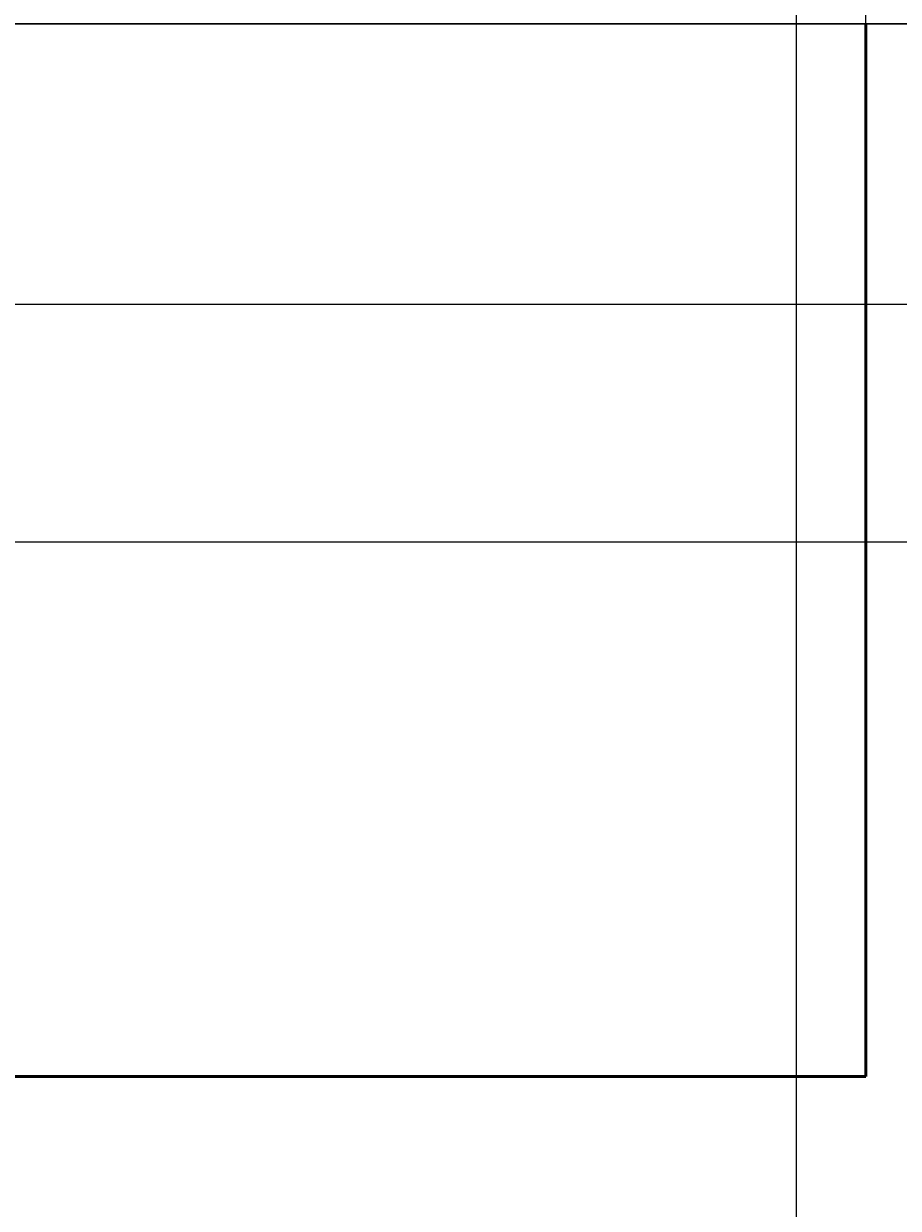
# Model space of a CAD drawing. Units: inches. Extents: x 37 to 824, y -700 to 234.
# Tile 64 of 77: x 314 to 364, y 8 to 75. Entities that reach past the tile are written whole.
import ezdxf

# ---------------------------------------------------------------- set-up
doc = ezdxf.new("R2010")
doc.units = ezdxf.units.IN
doc.header["$MEASUREMENT"] = 0
doc.layers.add('A-ANNO-DIMS', color=2, linetype='Continuous', lineweight=18)
doc.layers.add('A-WALL', color=2, linetype='Continuous', lineweight=50)
doc.styles.get("Standard").update_dxf_attribs({"font": 'arial.ttf'})
doc.dimstyles.get("Standard").update_dxf_attribs({"dimtxt": 0.18, "dimasz": 0.18, "dimexe": 0.18, "dimexo": 0.0625, "dimgap": 0.09, "dimtad": 0, "dimtih": 1, "dimtoh": 1, "dimdec": 1, "dimzin": 0, "dimdsep": 46, "dimlunit": 4, "dimtxsty": 'Standard', "dimcen": 0.09, "dimadec": 0, "dimazin": 0, "dimtfac": 1, "dimtdec": 1, "dimtofl": 0, "dimtmove": 0, "dimatfit": 3, "dimfxl": 1, "dimtolj": 1, "dimtzin": 0, "dimarcsym": 0})

# ---------------------------------------------------------------- blocks, each defined once
blk = doc.blocks.new('*D61')
at = {"layer": 'A-ANNO-DIMS', "color": 0, "lineweight": -2, "ltscale": 0.5, "transparency": 16777216}
for p, q in [((419.015, 75.09), (78.159, 75.09)), ((78.339, 74.91), (78.339, 67.271)), ((78.339, 59.27), (78.339, 66.91)), ((419.015, 59.09), (78.159, 59.09))]:
    blk.add_line(p, q, dxfattribs=at)
at = {"layer": 'A-ANNO-DIMS', "color": 0, "ltscale": 0.5, "transparency": 16777216}
for points in [[(78.309, 74.91), (78.369, 74.91), (78.339, 75.09)], [(78.309, 59.27), (78.369, 59.27), (78.339, 59.09)]]:
    blk.add_solid(points, dxfattribs=at)
at = {"layer": 'Defpoints', "color": 0, "ltscale": 0.5, "transparency": 16777216}
for p in [(419.077, 75.09), (78.339, 59.09), (419.077, 59.09)]:
    blk.add_point(p, dxfattribs=at)
at = {"layer": 'A-ANNO-DIMS', "color": 0, "ltscale": 0.5, "transparency": 16777216, "insert": (78.339, 67.09), "char_height": 0.18, "attachment_point": 5}
blk.add_mtext('\\A1;1\'-4"', dxfattribs=at)
blk = doc.blocks.new('*D76')
at = {"layer": 'A-ANNO-DIMS', "color": 0, "lineweight": -2, "ltscale": 0.5, "transparency": 16777216}
for p, q in [((227.14, 75.09), (513.773, 75.09)), ((513.593, 74.91), (513.593, 60.51)), ((513.593, 45.743), (513.593, 60.144)), ((227.14, 45.563), (513.773, 45.563))]:
    blk.add_line(p, q, dxfattribs=at)
at = {"layer": 'A-ANNO-DIMS', "color": 0, "ltscale": 0.5, "transparency": 16777216}
for points in [[(513.563, 74.91), (513.623, 74.91), (513.593, 75.09)], [(513.563, 45.743), (513.623, 45.743), (513.593, 45.563)]]:
    blk.add_solid(points, dxfattribs=at)
at = {"layer": 'Defpoints', "color": 0, "ltscale": 0.5, "transparency": 16777216}
for p in [(227.077, 75.09), (227.077, 45.563), (513.593, 45.563)]:
    blk.add_point(p, dxfattribs=at)
at = {"layer": 'A-ANNO-DIMS', "color": 0, "ltscale": 0.5, "transparency": 16777216, "insert": (513.593, 60.327), "char_height": 0.18, "attachment_point": 5}
blk.add_mtext('\\A1;2\'-5 1/2"', dxfattribs=at)
blk = doc.blocks.new('*D78')
at = {"layer": 'A-ANNO-DIMS', "color": 0, "lineweight": -2, "ltscale": 0.5, "transparency": 16777216}
for p, q in [((290.077, 15.153), (290.077, 234.17)), ((290.257, 233.99), (325.747, 233.99)), ((361.897, 233.99), (326.407, 233.99)), ((362.077, 15.153), (362.077, 234.17))]:
    blk.add_line(p, q, dxfattribs=at)
at = {"layer": 'A-ANNO-DIMS', "color": 0, "ltscale": 0.5, "transparency": 16777216}
for points in [[(290.257, 234.02), (290.257, 233.96), (290.077, 233.99)], [(361.897, 234.02), (361.897, 233.96), (362.077, 233.99)]]:
    blk.add_solid(points, dxfattribs=at)
at = {"layer": 'Defpoints', "color": 0, "ltscale": 0.5, "transparency": 16777216}
for p in [(362.077, 233.99), (290.077, 15.09), (362.077, 15.09)]:
    blk.add_point(p, dxfattribs=at)
at = {"layer": 'A-ANNO-DIMS', "color": 0, "ltscale": 0.5, "transparency": 16777216, "insert": (326.077, 233.99), "char_height": 0.18, "attachment_point": 5}
blk.add_mtext('\\A1;6\'-0"', dxfattribs=at)
blk = doc.blocks.new('*D82')
at = {"layer": 'A-ANNO-DIMS', "color": 0, "lineweight": -2, "ltscale": 0.5, "transparency": 16777216}
for p, q in [((299.077, -206.847), (299.077, 234.17)), ((299.257, 233.99), (328.202, 233.99)), ((357.952, 233.99), (329.008, 233.99)), ((358.132, -206.847), (358.132, 234.17))]:
    blk.add_line(p, q, dxfattribs=at)
at = {"layer": 'A-ANNO-DIMS', "color": 0, "ltscale": 0.5, "transparency": 16777216}
for points in [[(299.257, 234.02), (299.257, 233.96), (299.077, 233.99)], [(357.952, 234.02), (357.952, 233.96), (358.132, 233.99)]]:
    blk.add_solid(points, dxfattribs=at)
at = {"layer": 'Defpoints', "color": 0, "ltscale": 0.5, "transparency": 16777216}
for p in [(358.132, 233.99), (299.077, -206.91), (358.132, -206.91)]:
    blk.add_point(p, dxfattribs=at)
at = {"layer": 'A-ANNO-DIMS', "color": 0, "ltscale": 0.5, "transparency": 16777216, "insert": (328.605, 233.99), "char_height": 0.18, "attachment_point": 5}
blk.add_mtext('\\A1;4\'-11"', dxfattribs=at)
blk = doc.blocks.new('*D83')
at = {"layer": 'A-ANNO-DIMS', "color": 0, "lineweight": -2, "ltscale": 0.5, "transparency": 16777216}
for p, q in [((358.132, -206.847), (358.132, 234.17)), ((358.312, 233.99), (388.275, 233.99)), ((418.897, 233.99), (388.934, 233.99)), ((419.077, -206.847), (419.077, 234.17))]:
    blk.add_line(p, q, dxfattribs=at)
at = {"layer": 'A-ANNO-DIMS', "color": 0, "ltscale": 0.5, "transparency": 16777216}
for points in [[(358.312, 234.02), (358.312, 233.96), (358.132, 233.99)], [(418.897, 234.02), (418.897, 233.96), (419.077, 233.99)]]:
    blk.add_solid(points, dxfattribs=at)
at = {"layer": 'Defpoints', "color": 0, "ltscale": 0.5, "transparency": 16777216}
for p in [(419.077, 233.99), (358.132, -206.91), (419.077, -206.91)]:
    blk.add_point(p, dxfattribs=at)
at = {"layer": 'A-ANNO-DIMS', "color": 0, "ltscale": 0.5, "transparency": 16777216, "insert": (388.605, 233.99), "char_height": 0.18, "attachment_point": 5}
blk.add_mtext('\\A1;5\'-1"', dxfattribs=at)

msp = doc.modelspace()

# ---------------------------------------------------------------- linework, layer by layer
at = {"layer": 'A-WALL'}
for q in [(362.077, 75.09), (290.077, 15.09)]:
    msp.add_line((362.077, 15.09), q, dxfattribs=at)

# ---------------------------------------------------------------- dimensions: what is measured, and where the dimension line sits
at = {"layer": 'A-ANNO-DIMS', "ltscale": 0.5}
for base, p1, p2, picture, middle in [((362.077, 233.99), (290.077, 15.09), (362.077, 15.09), '*D78', (326.077, 233.99)), ((358.132, 233.99), (299.077, -206.91), (358.132, -206.91), '*D82', (328.605, 233.99)), ((419.077, 233.99), (358.132, -206.91), (419.077, -206.91), '*D83', (388.605, 233.99))]:
    dim = msp.add_linear_dim(base=base, p1=p1, p2=p2, dimstyle='Standard', override={"dimdec": 1, "dimlfac": 1, "dimrnd": 0, "dimzin": 1, "dimdsep": 46, "dimlunit": 4, "dimfrac": 2}, dxfattribs=at)
    dim.commit()
    dim.dimension.update_dxf_attribs({"geometry": picture, "text_midpoint": middle})
for base, p1, p2, picture, middle in [((78.339, 59.09), (419.077, 75.09), (419.077, 59.09), '*D61', (78.339, 67.09)), ((513.593, 45.563), (227.077, 75.09), (227.077, 45.563), '*D76', (513.593, 60.327))]:
    dim = msp.add_linear_dim(base=base, p1=p1, p2=p2, angle=90, dimstyle='Standard', override={"dimdec": 1, "dimlfac": 1, "dimrnd": 0, "dimzin": 1, "dimdsep": 46, "dimlunit": 4, "dimfrac": 2}, dxfattribs=at)
    dim.commit()
    dim.dimension.update_dxf_attribs({"geometry": picture, "text_midpoint": middle})

doc.saveas('drawing.dxf')
